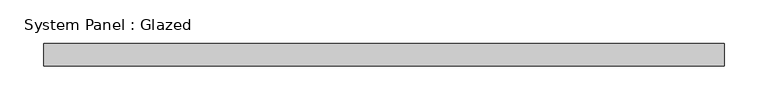
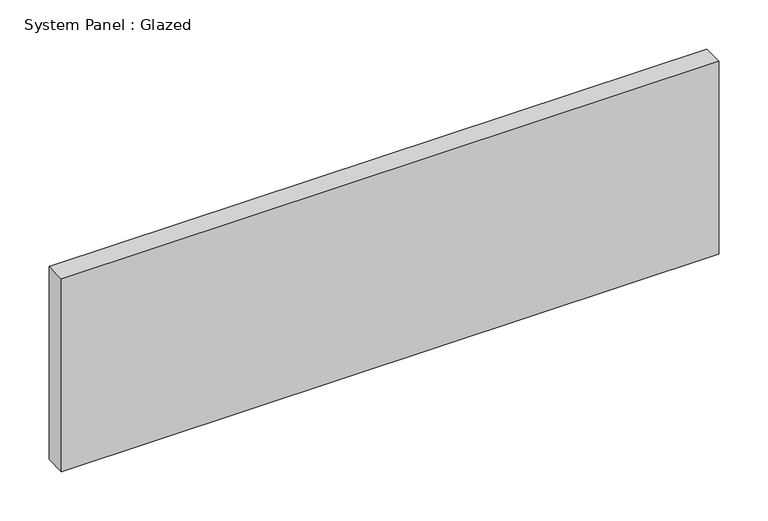
"""IFC4 building model written with IfcOpenShell, lengths in millimetres: plate geometry, System Panel : Glazed."""

from ifc_helpers import new_model, si_unit, origin, origin_with_axes, place, context, project, spatial, polyline, outline, extrude, source, transform, mapped, element, save


def system_panel_glazed_63219d49(model_context):
    return source(origin(), model_context, "Body", "SweptSolid", [
        extrude(outline(polyline([(387.35, 19.05), (-387.35, 19.05), (-387.35, 44.45), (387.35, 44.45), (387.35, 19.05)])), origin_with_axes(), (0.0, 0.0, 1.0), 240.4951523),
    ])


if __name__ == "__main__":
    model = new_model("IFC4")
    model_context = context("Model", 3, world=origin())
    ifc_project = project(units=[si_unit("LENGTHUNIT", "METRE", prefix="MILLI")], contexts=[model_context])
    site = spatial("IfcSite", under=ifc_project)
    building = spatial("IfcBuilding", under=site)
    placement = place(None, origin())
    system_panel_glazed_shape = system_panel_glazed_63219d49(model_context)
    element("IfcPlate", 1, ObjectType="System Panel : Glazed", at=placement, inside=building, context=model_context, shape_type="MappedRepresentation", body=[
        mapped(system_panel_glazed_shape, transform((0.0, 0.0, 0.0), x_axis=(1.0, 0.0, 0.0), y_axis=(0.0, 1.0, 0.0), z_axis=(0.0, 0.0, 1.0))),
    ])
    save(model, "model.ifc")

# Revit data of these elements
# Type "System Panel : Glazed"
#   Construction Type Id = "GSP4R"
#   Analytic Construction = "1/8 in Pilkington single glazing"
#   Visual Light Transmittance = 0.9
#   Solar Heat Gain Coefficient = 0.86
#   Heat Transfer Coefficient (U) = 1.18115 BTU/(h·ft²·°F)
#   Define Thermal Properties by = 1
# Element 1 (IfcPlate, "System Panel : Glazed")
#   Materials on its faces: "Glass"
# Materials
#   "Glass": class "Glass", colour RGB 0 128 192, transparency 0.75, Description = "Soda Lime Glass", Cost = 0
